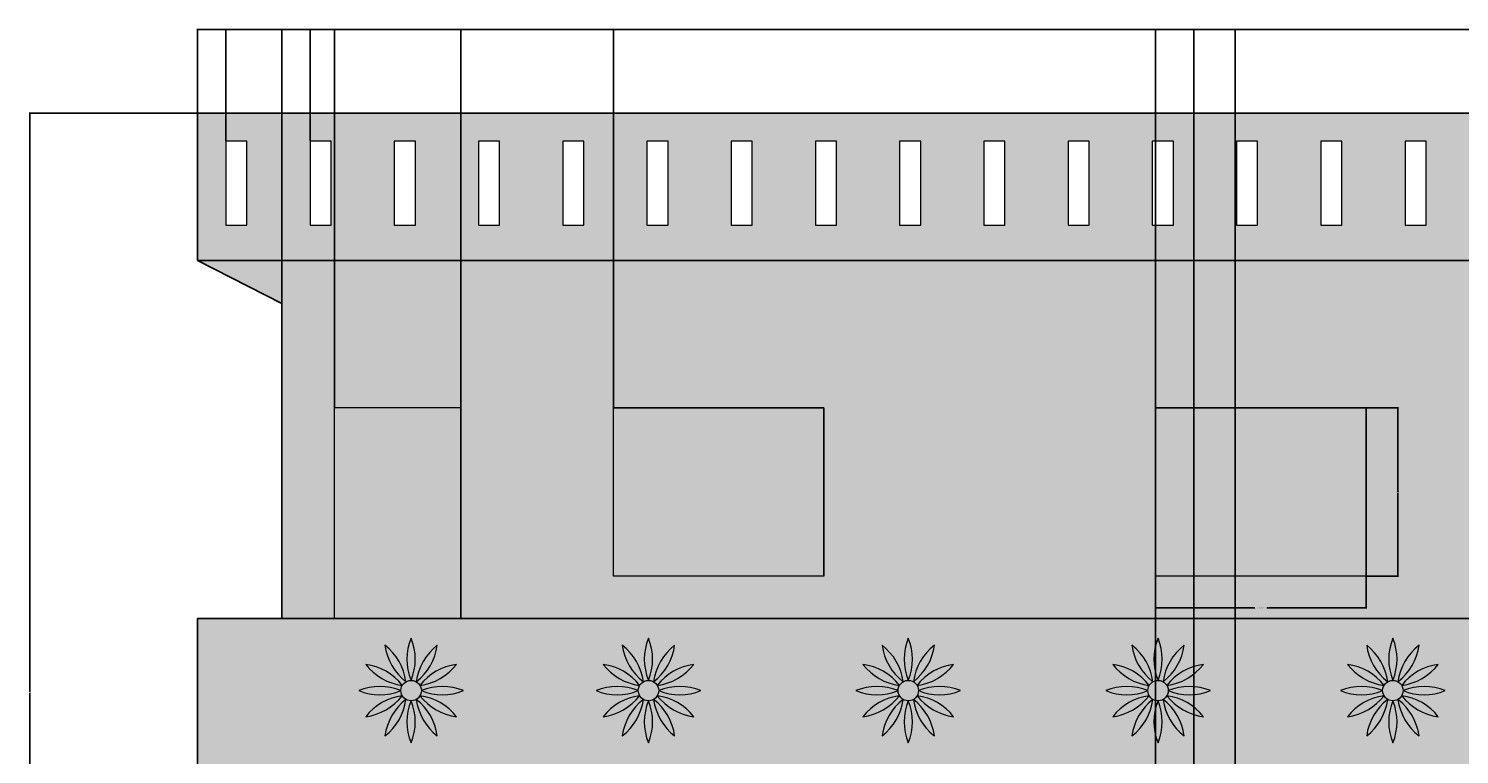
# Model space of a CAD drawing. Units: inches. Extents: x -43 to 1296, y -568 to 542.
# Tile 6 of 14: x -43 to 364, y 336 to 542. Entities that reach past the tile are written whole.
import ezdxf

# ---------------------------------------------------------------- set-up
doc = ezdxf.new("R2010")
doc.units = ezdxf.units.IN
doc.header["$MEASUREMENT"] = 0
for name, color, linetype, lineweight in [('A-ANNO-DIMS', 2, 'Continuous', 18), ('A-DOOR', 3, 'Continuous', 18), ('A-ELEV', 7, 'Continuous', 25), ('A-ELEV-OPEN-PATT', 13, 'Continuous', 13), ('A-ELEV-TRIM', 7, 'Continuous', 18), ('A-ELEV-TRIM-PATT', 4, 'Continuous', 13), ('A-GLAZ-ELEV', 4, 'Continuous', 18)]:
    doc.layers.add(name, color=color, linetype=linetype, lineweight=lineweight)
for name, color, linetype, lineweight, true_color in [('A-ELEV-BAND-PATT', 30, 'Continuous', 13, 0xf8991e), ('A-ELEV-WALL-PATT', 31, 'Continuous', 13, 0xfecc66), ('A-ROOF-PATT', 217, 'Continuous', 13, 0x93278f)]:
    doc.layers.add(name, color=color, linetype=linetype, lineweight=lineweight, true_color=true_color)
doc.styles.get("Standard").update_dxf_attribs({"font": 'arial.ttf'})
doc.dimstyles.get("Standard").update_dxf_attribs({"dimtxt": 0.18, "dimasz": 0.18, "dimexe": 0.18, "dimexo": 0.0625, "dimgap": 0.09, "dimtad": 0, "dimtih": 1, "dimtoh": 1, "dimdec": 0, "dimzin": 0, "dimdsep": 46, "dimlunit": 3, "dimtxsty": 'Standard', "dimcen": 0.09, "dimadec": 0, "dimazin": 0, "dimtfac": 1, "dimtdec": 0, "dimtofl": 0, "dimtmove": 0, "dimatfit": 3, "dimfxl": 1, "dimtolj": 1, "dimtzin": 0, "dimarcsym": 0})

# ---------------------------------------------------------------- blocks, each defined once
blk = doc.blocks.new('*U5')
for p, q in [((-3, 12), (-3, -12)), ((3, 12), (-3, 12)), ((3, -12), (3, 12)), ((-3, -12), (3, -12))]:
    blk.add_line(p, q)
blk = doc.blocks.new('*U6')
at = {"layer": 'A-ELEV-TRIM', "color": 0, "linetype": 'ByBlock', "lineweight": -2, "transparency": 16777216}
for p in [(0, 0), (24, 0), (48, 0), (72, 0), (96, 0), (120, 0), (144, 0), (168, 0), (192, 0), (216, 0), (240, 0), (264, 0), (288, 0), (312, 0), (336, 0), (360, 0), (384, 0)]:
    blk.add_blockref('*U5', p, dxfattribs=at)
blk = doc.blocks.new('*U9')
for centre, start, end in [((14.57, 0), 157.6165, 202.3835), ((-14.57, 0), 337.6165, 22.3835)]:
    blk.add_arc(centre, 15.76, start, end)
blk = doc.blocks.new('*U10')
at = {"layer": 'A-ELEV-TRIM', "color": 0, "linetype": 'ByBlock', "lineweight": -2, "transparency": 16777216}
for p, rotation in [((202.9, 361.45), 29.99999999999998), ((211.82, 361.45), 329.9999999999999), ((199.64, 358.19), 59.99999999999999), ((215.08, 358.19), 300), ((198.44, 353.73), 90), ((216.28, 353.73), 269.9999999999999), ((199.64, 349.27), 120), ((202.9, 346.01), 150), ((207.36, 344.81), 180), ((211.82, 346.01), 210), ((215.08, 349.27), 240)]:
    blk.add_blockref('*U9', p, dxfattribs=dict(at, rotation=rotation))
blk.add_blockref('*U9', (207.36, 362.65), dxfattribs=at)
blk = doc.blocks.new('*U11')
for centre, start, end in [((14.57, 0), 157.6165, 202.3835), ((-14.57, 0), 337.6165, 22.3835)]:
    blk.add_arc(centre, 15.76, start, end)
blk = doc.blocks.new('*U12')
at = {"layer": 'A-ELEV-TRIM', "color": 0, "linetype": 'ByBlock', "lineweight": -2, "transparency": 16777216}
for p, rotation in [((202.9, 361.45), 29.99999999999998), ((211.82, 361.45), 329.9999999999999), ((199.64, 358.19), 59.99999999999999), ((215.08, 358.19), 300), ((198.44, 353.73), 90), ((216.28, 353.73), 269.9999999999999), ((199.64, 349.27), 120), ((202.9, 346.01), 150), ((207.36, 344.81), 180), ((211.82, 346.01), 210), ((215.08, 349.27), 240)]:
    blk.add_blockref('*U11', p, dxfattribs=dict(at, rotation=rotation))
blk.add_blockref('*U11', (207.36, 362.65), dxfattribs=at)
blk = doc.blocks.new('*U13')
for centre, start, end in [((14.57, 0), 157.6165, 202.3835), ((-14.57, 0), 337.6165, 22.3835)]:
    blk.add_arc(centre, 15.76, start, end)
blk = doc.blocks.new('*U14')
at = {"layer": 'A-ELEV-TRIM', "color": 0, "linetype": 'ByBlock', "lineweight": -2, "transparency": 16777216}
for p, rotation in [((202.9, 361.45), 29.99999999999998), ((211.82, 361.45), 329.9999999999999), ((199.64, 358.19), 59.99999999999999), ((215.08, 358.19), 300), ((198.44, 353.73), 90), ((216.28, 353.73), 269.9999999999999), ((199.64, 349.27), 120), ((202.9, 346.01), 150), ((207.36, 344.81), 180), ((211.82, 346.01), 210), ((215.08, 349.27), 240)]:
    blk.add_blockref('*U13', p, dxfattribs=dict(at, rotation=rotation))
blk.add_blockref('*U13', (207.36, 362.65), dxfattribs=at)
blk = doc.blocks.new('*U15')
for centre, start, end in [((14.57, 0), 157.6165, 202.3835), ((-14.57, 0), 337.6165, 22.3835)]:
    blk.add_arc(centre, 15.76, start, end)
blk = doc.blocks.new('*U16')
at = {"layer": 'A-ELEV-TRIM', "color": 0, "linetype": 'ByBlock', "lineweight": -2, "transparency": 16777216}
for p, rotation in [((202.9, 361.45), 29.99999999999998), ((211.82, 361.45), 329.9999999999999), ((199.64, 358.19), 59.99999999999999), ((215.08, 358.19), 300), ((198.44, 353.73), 90), ((216.28, 353.73), 269.9999999999999), ((199.64, 349.27), 120), ((202.9, 346.01), 150), ((207.36, 344.81), 180), ((211.82, 346.01), 210), ((215.08, 349.27), 240)]:
    blk.add_blockref('*U15', p, dxfattribs=dict(at, rotation=rotation))
blk.add_blockref('*U15', (207.36, 362.65), dxfattribs=at)
blk = doc.blocks.new('*U17')
for centre, start, end in [((14.57, 0), 157.6165, 202.3835), ((-14.57, 0), 337.6165, 22.3835)]:
    blk.add_arc(centre, 15.76, start, end)
blk = doc.blocks.new('*U18')
at = {"layer": 'A-ELEV-TRIM', "color": 0, "linetype": 'ByBlock', "lineweight": -2, "transparency": 16777216}
for p, rotation in [((202.9, 361.45), 29.99999999999998), ((211.82, 361.45), 329.9999999999999), ((199.64, 358.19), 59.99999999999999), ((215.08, 358.19), 300), ((198.44, 353.73), 90), ((216.28, 353.73), 269.9999999999999), ((199.64, 349.27), 120), ((202.9, 346.01), 150), ((207.36, 344.81), 180), ((211.82, 346.01), 210), ((215.08, 349.27), 240)]:
    blk.add_blockref('*U17', p, dxfattribs=dict(at, rotation=rotation))
blk.add_blockref('*U17', (207.36, 362.65), dxfattribs=at)
blk = doc.blocks.new('WIN-ELEV-60x48')
for p, q in [((60, 48), (0, 48)), ((0, 0), (0, 48)), ((60, 0), (60, 48)), ((60, 0), (0, 0))]:
    blk.add_line(p, q)
blk = doc.blocks.new('*D52')
at = {"layer": 'A-ANNO-DIMS', "color": 0, "lineweight": -2, "transparency": 16777216}
for p, q in [((277.84, 386.23), (277.84, 377.11)), ((337.84, 386.23), (337.84, 377.11)), ((278.02, 377.29), (306.15, 377.29)), ((337.66, 377.29), (309.53, 377.29))]:
    blk.add_line(p, q, dxfattribs=at)
at = {"layer": 'A-ANNO-DIMS', "color": 0, "transparency": 16777216}
for points in [[(278.02, 377.32), (278.02, 377.26), (277.84, 377.29)], [(337.66, 377.32), (337.66, 377.26), (337.84, 377.29)]]:
    blk.add_solid(points, dxfattribs=at)
at = {"layer": 'Defpoints', "color": 0, "transparency": 16777216}
for p in [(277.84, 386.29), (337.84, 386.29), (337.84, 377.29)]:
    blk.add_point(p, dxfattribs=at)
at = {"layer": 'A-ANNO-DIMS', "color": 0, "transparency": 16777216, "insert": (307.84, 377.29), "char_height": 0.18, "attachment_point": 5}
blk.add_mtext('\\A1;UPPER WINDOW 5\'-0" TYP.', dxfattribs=at)
blk = doc.blocks.new('*D53')
at = {"layer": 'A-ANNO-DIMS', "color": 0, "lineweight": -2, "transparency": 16777216}
for p, q in [((337.91, 434.29), (347.02, 434.29)), ((346.84, 434.11), (346.84, 410.47)), ((346.84, 386.47), (346.84, 410.11)), ((337.91, 386.29), (347.02, 386.29))]:
    blk.add_line(p, q, dxfattribs=at)
at = {"layer": 'A-ANNO-DIMS', "color": 0, "transparency": 16777216}
for points in [[(346.81, 434.11), (346.87, 434.11), (346.84, 434.29)], [(346.81, 386.47), (346.87, 386.47), (346.84, 386.29)]]:
    blk.add_solid(points, dxfattribs=at)
at = {"layer": 'Defpoints', "color": 0, "transparency": 16777216}
for p in [(337.84, 434.29), (346.84, 434.29), (337.84, 386.29)]:
    blk.add_point(p, dxfattribs=at)
at = {"layer": 'A-ANNO-DIMS', "color": 0, "transparency": 16777216, "insert": (346.84, 410.29), "char_height": 0.18, "attachment_point": 5}
blk.add_mtext('\\A1;4\'-0" TYP.', dxfattribs=at)
blk = doc.blocks.new('*D61')
at = {"layer": 'A-ANNO-DIMS', "color": 0, "lineweight": -2, "transparency": 16777216}
for p, q in [((4.78, 518.29), (-43.14, 518.29)), ((-42.96, 518.11), (-42.96, 353.47)), ((-42.96, 188.47), (-42.96, 353.11)), ((-19.22, 188.29), (-43.14, 188.29))]:
    blk.add_line(p, q, dxfattribs=at)
at = {"layer": 'A-ANNO-DIMS', "color": 0, "transparency": 16777216}
for points in [[(-42.99, 518.11), (-42.93, 518.11), (-42.96, 518.29)], [(-42.99, 188.47), (-42.93, 188.47), (-42.96, 188.29)]]:
    blk.add_solid(points, dxfattribs=at)
at = {"layer": 'Defpoints', "color": 0, "transparency": 16777216}
for p in [(-42.96, 518.29), (4.84, 518.29), (-19.16, 188.29)]:
    blk.add_point(p, dxfattribs=at)
at = {"layer": 'A-ANNO-DIMS', "color": 0, "transparency": 16777216, "insert": (-42.96, 353.29), "char_height": 0.18, "attachment_point": 5}
blk.add_mtext('\\A1;27\'-6"', dxfattribs=at)
blk = doc.blocks.new('*D70')
at = {"layer": 'A-ANNO-DIMS', "color": 0, "lineweight": -2, "transparency": 16777216}
for p, q in [((277.84, 188.35), (277.84, 542.27)), ((288.75, 188.35), (288.75, 542.27)), ((278.02, 542.09), (282.89, 542.09)), ((288.57, 542.09), (283.69, 542.09))]:
    blk.add_line(p, q, dxfattribs=at)
at = {"layer": 'A-ANNO-DIMS', "color": 0, "transparency": 16777216}
for points in [[(278.02, 542.12), (278.02, 542.06), (277.84, 542.09)], [(288.57, 542.12), (288.57, 542.06), (288.75, 542.09)]]:
    blk.add_solid(points, dxfattribs=at)
at = {"layer": 'Defpoints', "color": 0, "transparency": 16777216}
for p in [(288.75, 542.09), (277.84, 188.29), (288.75, 188.29)]:
    blk.add_point(p, dxfattribs=at)
at = {"layer": 'A-ANNO-DIMS', "color": 0, "transparency": 16777216, "insert": (283.29, 542.09), "char_height": 0.18, "attachment_point": 5}
blk.add_mtext('\\A1;0\'-11"', dxfattribs=at)
blk = doc.blocks.new('*D71')
at = {"layer": 'A-ANNO-DIMS', "color": 0, "lineweight": -2, "transparency": 16777216}
for p, q in [((288.75, 235.13), (288.75, 542.27)), ((300.49, 239.65), (300.49, 542.27)), ((288.93, 542.09), (294.01, 542.09)), ((300.31, 542.09), (295.23, 542.09))]:
    blk.add_line(p, q, dxfattribs=at)
at = {"layer": 'A-ANNO-DIMS', "color": 0, "transparency": 16777216}
for points in [[(288.93, 542.12), (288.93, 542.06), (288.75, 542.09)], [(300.31, 542.12), (300.31, 542.06), (300.49, 542.09)]]:
    blk.add_solid(points, dxfattribs=at)
at = {"layer": 'Defpoints', "color": 0, "transparency": 16777216}
for p in [(300.49, 542.09), (300.49, 239.58), (288.75, 235.07)]:
    blk.add_point(p, dxfattribs=at)
at = {"layer": 'A-ANNO-DIMS', "color": 0, "transparency": 16777216, "insert": (294.62, 542.09), "char_height": 0.18, "attachment_point": 5}
blk.add_mtext('\\A1;0\'-11 1/2"', dxfattribs=at)
blk = doc.blocks.new('*D73')
at = {"layer": 'A-ANNO-DIMS', "color": 0, "lineweight": -2, "transparency": 16777216}
for p, q in [((4.84, 518.35), (4.84, 542.27)), ((412.84, 518.35), (412.84, 542.27)), ((5.02, 542.09), (208.44, 542.09)), ((412.66, 542.09), (209.24, 542.09))]:
    blk.add_line(p, q, dxfattribs=at)
at = {"layer": 'A-ANNO-DIMS', "color": 0, "transparency": 16777216}
for points in [[(5.02, 542.12), (5.02, 542.06), (4.84, 542.09)], [(412.66, 542.12), (412.66, 542.06), (412.84, 542.09)]]:
    blk.add_solid(points, dxfattribs=at)
at = {"layer": 'Defpoints', "color": 0, "transparency": 16777216}
for p in [(412.84, 542.09), (4.84, 518.29), (412.84, 518.29)]:
    blk.add_point(p, dxfattribs=at)
at = {"layer": 'A-ANNO-DIMS', "color": 0, "transparency": 16777216, "insert": (208.84, 542.09), "char_height": 0.18, "attachment_point": 5}
blk.add_mtext('\\A1;34\'-0"', dxfattribs=at)
blk = doc.blocks.new('*D74')
at = {"layer": 'A-ANNO-DIMS', "color": 0, "lineweight": -2, "transparency": 16777216}
for p, q in [((28.84, 476.35), (28.84, 542.27)), ((43.84, 434.35), (43.84, 542.27)), ((29.02, 542.09), (36.02, 542.09)), ((43.66, 542.09), (36.66, 542.09))]:
    blk.add_line(p, q, dxfattribs=at)
at = {"layer": 'A-ANNO-DIMS', "color": 0, "transparency": 16777216}
for points in [[(29.02, 542.12), (29.02, 542.06), (28.84, 542.09)], [(43.66, 542.12), (43.66, 542.06), (43.84, 542.09)]]:
    blk.add_solid(points, dxfattribs=at)
at = {"layer": 'Defpoints', "color": 0, "transparency": 16777216}
for p in [(43.84, 542.09), (28.84, 476.29), (43.84, 434.29)]:
    blk.add_point(p, dxfattribs=at)
at = {"layer": 'A-ANNO-DIMS', "color": 0, "transparency": 16777216, "insert": (36.34, 542.09), "char_height": 0.18, "attachment_point": 5}
blk.add_mtext('\\A1;1\'-3"', dxfattribs=at)
blk = doc.blocks.new('*D75')
at = {"layer": 'A-ANNO-DIMS', "color": 0, "lineweight": -2, "transparency": 16777216}
for p, q in [((43.84, 434.35), (43.84, 542.27)), ((79.84, 434.35), (79.84, 542.27)), ((44.02, 542.09), (61.51, 542.09)), ((79.66, 542.09), (62.17, 542.09))]:
    blk.add_line(p, q, dxfattribs=at)
at = {"layer": 'A-ANNO-DIMS', "color": 0, "transparency": 16777216}
for points in [[(44.02, 542.12), (44.02, 542.06), (43.84, 542.09)], [(79.66, 542.12), (79.66, 542.06), (79.84, 542.09)]]:
    blk.add_solid(points, dxfattribs=at)
at = {"layer": 'Defpoints', "color": 0, "transparency": 16777216}
for p in [(79.84, 542.09), (43.84, 434.29), (79.84, 434.29)]:
    blk.add_point(p, dxfattribs=at)
at = {"layer": 'A-ANNO-DIMS', "color": 0, "transparency": 16777216, "insert": (61.84, 542.09), "char_height": 0.18, "attachment_point": 5}
blk.add_mtext('\\A1;3\'-0"', dxfattribs=at)
blk = doc.blocks.new('*D76')
at = {"layer": 'A-ANNO-DIMS', "color": 0, "lineweight": -2, "transparency": 16777216}
for p, q in [((79.84, 434.35), (79.84, 542.27)), ((123.34, 434.35), (123.34, 542.27)), ((80.02, 542.09), (101.05, 542.09)), ((123.16, 542.09), (102.13, 542.09))]:
    blk.add_line(p, q, dxfattribs=at)
at = {"layer": 'A-ANNO-DIMS', "color": 0, "transparency": 16777216}
for points in [[(80.02, 542.12), (80.02, 542.06), (79.84, 542.09)], [(123.16, 542.12), (123.16, 542.06), (123.34, 542.09)]]:
    blk.add_solid(points, dxfattribs=at)
at = {"layer": 'Defpoints', "color": 0, "transparency": 16777216}
for p in [(123.34, 542.09), (79.84, 434.29), (123.34, 434.29)]:
    blk.add_point(p, dxfattribs=at)
at = {"layer": 'A-ANNO-DIMS', "color": 0, "transparency": 16777216, "insert": (101.59, 542.09), "char_height": 0.18, "attachment_point": 5}
blk.add_mtext('\\A1;3\'-7 1/2"', dxfattribs=at)
blk = doc.blocks.new('*D77')
at = {"layer": 'A-ANNO-DIMS', "color": 0, "lineweight": -2, "transparency": 16777216}
for p, q in [((123.34, 434.35), (123.34, 542.27)), ((277.84, 434.35), (277.84, 542.27)), ((123.52, 542.09), (199.92, 542.09)), ((277.66, 542.09), (201.26, 542.09))]:
    blk.add_line(p, q, dxfattribs=at)
at = {"layer": 'A-ANNO-DIMS', "color": 0, "transparency": 16777216}
for points in [[(123.52, 542.12), (123.52, 542.06), (123.34, 542.09)], [(277.66, 542.12), (277.66, 542.06), (277.84, 542.09)]]:
    blk.add_solid(points, dxfattribs=at)
at = {"layer": 'Defpoints', "color": 0, "transparency": 16777216}
for p in [(277.84, 542.09), (123.34, 434.29), (277.84, 434.29)]:
    blk.add_point(p, dxfattribs=at)
at = {"layer": 'A-ANNO-DIMS', "color": 0, "transparency": 16777216, "insert": (200.59, 542.09), "char_height": 0.18, "attachment_point": 5}
blk.add_mtext('\\A1;12\'-10 1/2"', dxfattribs=at)
blk = doc.blocks.new('*D78')
at = {"layer": 'A-ANNO-DIMS', "color": 0, "lineweight": -2, "transparency": 16777216}
for p, q in [((12.9, 510.38), (12.9, 542.27)), ((36.9, 510.38), (36.9, 542.27)), ((13.08, 542.09), (24.57, 542.09)), ((36.72, 542.09), (25.23, 542.09))]:
    blk.add_line(p, q, dxfattribs=at)
at = {"layer": 'A-ANNO-DIMS', "color": 0, "transparency": 16777216}
for points in [[(13.08, 542.12), (13.08, 542.06), (12.9, 542.09)], [(36.72, 542.12), (36.72, 542.06), (36.9, 542.09)]]:
    blk.add_solid(points, dxfattribs=at)
at = {"layer": 'Defpoints', "color": 0, "transparency": 16777216}
for p in [(36.9, 542.09), (12.9, 510.31), (36.9, 510.31)]:
    blk.add_point(p, dxfattribs=at)
at = {"layer": 'A-ANNO-DIMS', "color": 0, "transparency": 16777216, "insert": (24.9, 542.09), "char_height": 0.18, "attachment_point": 5}
blk.add_mtext('\\A1;2\'-0"', dxfattribs=at)

msp = doc.modelspace()

# ---------------------------------------------------------------- hatches: boundary and pattern name
at = {"layer": 'A-ELEV-BAND-PATT'}
h = msp.add_hatch(color=256, dxfattribs=at)
h.dxf.hatch_style = 1
h.paths.add_polyline_path([(412.84, 374.29), (4.84, 374.29), (4.84, 332.29), (412.84, 332.29)])
h.paths.add_polyline_path([(222.28, 353.73, -0.197856), (210.28, 353.73, -0.131652), (209.89, 352.27, -0.197856), (220.28, 346.27, -0.197856), (209.89, 352.27, -0.131652), (208.82, 351.2, -0.197856), (214.82, 340.81, -0.197856), (208.82, 351.2, -0.131652), (207.36, 350.81, -0.197856), (207.36, 338.81, -0.197856), (207.36, 350.81, -0.131652), (205.9, 351.2, -0.197856), (199.9, 340.81, -0.197856), (205.9, 351.2, -0.131652), (204.83, 352.27, -0.197856), (194.44, 346.27, -0.197856), (204.83, 352.27, -0.131652), (204.44, 353.73, -0.197856), (192.44, 353.73, -0.197856), (204.44, 353.73, -0.131652), (204.83, 355.19, -0.197856), (194.44, 361.19, -0.197856), (204.83, 355.19, -0.131652), (205.9, 356.25, -0.197856), (199.9, 366.65, -0.197856), (205.9, 356.25, -0.131652), (207.36, 356.65, -0.197856), (207.36, 368.65, -0.197856), (207.36, 356.65, -0.131652), (208.82, 356.25, -0.197856), (214.82, 366.65, -0.197856), (208.82, 356.25, -0.131652), (209.89, 355.19, -0.197856), (220.28, 361.19, -0.197856), (209.89, 355.19, -0.131652), (210.28, 353.73, -0.197856)], flags=16)
h.paths.add_polyline_path([(263.61, 353.73, -0.197856), (275.61, 353.73, -0.131652), (276, 355.19, -0.197856), (265.61, 361.19, -0.197856), (276, 355.19, -0.131652), (277.07, 356.25, -0.197856), (271.07, 366.65, -0.197856), (277.07, 356.25, -0.131652), (278.53, 356.65, -0.197856), (278.53, 368.65, -0.197856), (278.53, 356.65, -0.131652), (279.99, 356.25, -0.197856), (285.99, 366.65, -0.197856), (279.99, 356.25, -0.131652), (281.06, 355.19, -0.197856), (291.45, 361.19, -0.197856), (281.06, 355.19, -0.131652), (281.45, 353.73, -0.197856), (293.45, 353.73, -0.197856), (281.45, 353.73, -0.131652), (281.06, 352.27, -0.197856), (291.45, 346.27, -0.197856), (281.06, 352.27, -0.131652), (279.99, 351.2, -0.197856), (285.99, 340.81, -0.197856), (279.99, 351.2, -0.131652), (278.53, 350.81, -0.197856), (278.53, 338.81, -0.197856), (278.53, 350.81, -0.131652), (277.07, 351.2, -0.197856), (271.07, 340.81, -0.197856), (277.07, 351.2, -0.131652), (276, 352.27, -0.197856), (265.61, 346.27, -0.197856), (276, 352.27, -0.131652), (275.61, 353.73, -0.197856)], flags=16)
h.paths.add_polyline_path([(330.52, 353.73, -0.197856), (342.52, 353.73, -0.131652), (342.91, 355.19, -0.197856), (332.52, 361.19, -0.197856), (342.91, 355.19, -0.131652), (343.98, 356.25, -0.197856), (337.98, 366.65, -0.197856), (343.98, 356.25, -0.131652), (345.44, 356.65, -0.197856), (345.44, 368.65, -0.197856), (345.44, 356.65, -0.131652), (346.9, 356.25, -0.197856), (352.9, 366.65, -0.197856), (346.9, 356.25, -0.131652), (347.97, 355.19, -0.197856), (358.36, 361.19, -0.197856), (347.97, 355.19, -0.131652), (348.36, 353.73, -0.197856), (360.36, 353.73, -0.197856), (348.36, 353.73, -0.131652), (347.97, 352.27, -0.197856), (358.36, 346.27, -0.197856), (347.97, 352.27, -0.131652), (346.9, 351.2, -0.197856), (352.9, 340.81, -0.197856), (346.9, 351.2, -0.131652), (345.44, 350.81, -0.197856), (345.44, 338.81, -0.197856), (345.44, 350.81, -0.131652), (343.98, 351.2, -0.197856), (337.98, 340.81, -0.197856), (343.98, 351.2, -0.131652), (342.91, 352.27, -0.197856), (332.52, 346.27, -0.197856), (342.91, 352.27, -0.131652), (342.52, 353.73, -0.197856)], flags=16)
h.paths.add_polyline_path([(148.25, 353.73, -0.197856), (136.25, 353.73, -0.131652), (135.85, 352.27, -0.197856), (146.25, 346.27, -0.197856), (135.85, 352.27, -0.131652), (134.79, 351.2, -0.197856), (140.79, 340.81, -0.197856), (134.79, 351.2, -0.131652), (133.33, 350.81, -0.197856), (133.33, 338.81, -0.197856), (133.33, 350.81, -0.131652), (131.87, 351.2, -0.197856), (125.87, 340.81, -0.197856), (131.87, 351.2, -0.131652), (130.8, 352.27, -0.197856), (120.41, 346.27, -0.197856), (130.8, 352.27, -0.131652), (130.41, 353.73, -0.197856), (118.41, 353.73, -0.197856), (130.41, 353.73, -0.131652), (130.8, 355.19, -0.197856), (120.41, 361.19, -0.197856), (130.8, 355.19, -0.131652), (131.87, 356.25, -0.197856), (125.87, 366.65, -0.197856), (131.87, 356.25, -0.131652), (133.33, 356.65, -0.197856), (133.33, 368.65, -0.197856), (133.33, 356.65, -0.131652), (134.79, 356.25, -0.197856), (140.79, 366.65, -0.197856), (134.79, 356.25, -0.131652), (135.85, 355.19, -0.197856), (146.25, 361.19, -0.197856), (135.85, 355.19, -0.131652), (136.25, 353.73, -0.197856)], flags=16)
h.paths.add_polyline_path([(80.61, 353.73, -0.197856), (68.61, 353.73, -0.131652), (68.22, 352.27, -0.197856), (78.61, 346.27, -0.197856), (68.22, 352.27, -0.131652), (67.15, 351.2, -0.197856), (73.15, 340.81, -0.197856), (67.15, 351.2, -0.131652), (65.69, 350.81, -0.197856), (65.69, 338.81, -0.197856), (65.69, 350.81, -0.131652), (64.23, 351.2, -0.197856), (58.23, 340.81, -0.197856), (64.23, 351.2, -0.131652), (63.16, 352.27, -0.197856), (52.77, 346.27, -0.197856), (63.16, 352.27, -0.131652), (62.77, 353.73, -0.197856), (50.77, 353.73, -0.197856), (62.77, 353.73, -0.131652), (63.16, 355.19, -0.197856), (52.77, 361.19, -0.197856), (63.16, 355.19, -0.131652), (64.23, 356.25, -0.197856), (58.23, 366.65, -0.197856), (64.23, 356.25, -0.131652), (65.69, 356.65, -0.197856), (65.69, 368.65, -0.197856), (65.69, 356.65, -0.131652), (67.15, 356.25, -0.197856), (73.15, 366.65, -0.197856), (67.15, 356.25, -0.131652), (68.22, 355.19, -0.197856), (78.61, 361.19, -0.197856), (68.22, 355.19, -0.131652), (68.61, 353.73, -0.197856)], flags=16)
at = {"layer": 'A-ELEV-OPEN-PATT'}
h = msp.add_hatch(color=256, dxfattribs=at)
h.dxf.hatch_style = 1
h.paths.add_polyline_path([(79.84, 434.29), (43.84, 434.29), (43.84, 374.29), (79.84, 374.29)])
h.paths.add_polyline_path([(183.34, 434.29), (123.34, 434.29), (123.34, 386.29), (183.34, 386.29)])
h.paths.add_polyline_path([(337.84, 434.29), (277.84, 434.29), (277.84, 386.29), (337.84, 386.29)])
h.paths.add_polyline_path([(79.84, 290.29), (43.84, 290.29), (43.84, 248.29), (79.84, 248.29)])
h.paths.add_polyline_path([(183.34, 290.29), (123.34, 290.29), (123.34, 248.29), (183.34, 248.29)])
h.paths.add_polyline_path([(337.84, 290.29), (277.84, 290.29), (277.84, 248.29), (277.84, 230.87), (323.14, 248.29), (337.84, 242.64), (337.84, 248.29)])
h.paths.add_polyline_path([(1016.13, 374.59), (980.13, 374.59), (980.13, 290.59), (1016.13, 290.59)])
h.paths.add_polyline_path([(1016.13, 230.59), (980.13, 230.59), (980.13, 146.59), (1016.13, 146.59)])
h.paths.add_polyline_path([(833.13, 374.59), (824.13, 374.59), (824.13, 326.59), (833.13, 326.59)])
h.paths.add_polyline_path([(833.13, 230.59), (824.13, 230.59), (824.13, 182.59), (833.13, 182.59)])
at = {"layer": 'A-ELEV-TRIM-PATT'}
h = msp.add_hatch(color=256, dxfattribs=at)
h.dxf.hatch_style = 1
h.paths.add_polyline_path([(222.28, 353.73, -0.197856), (210.28, 353.73, -0.131652), (209.89, 352.27, -0.197856), (220.28, 346.27, -0.197856), (209.89, 352.27, -0.131652), (208.82, 351.2, -0.197856), (214.82, 340.81, -0.197856), (208.82, 351.2, -0.131652), (207.36, 350.81, -0.197856), (207.36, 338.81, -0.197856), (207.36, 350.81, -0.131652), (205.9, 351.2, -0.197856), (199.9, 340.81, -0.197856), (205.9, 351.2, -0.131652), (204.83, 352.27, -0.197856), (194.44, 346.27, -0.197856), (204.83, 352.27, -0.131652), (204.44, 353.73, -0.197856), (192.44, 353.73, -0.197856), (204.44, 353.73, -0.131652), (204.83, 355.19, -0.197856), (194.44, 361.19, -0.197856), (204.83, 355.19, -0.131652), (205.9, 356.25, -0.197856), (199.9, 366.65, -0.197856), (205.9, 356.25, -0.131652), (207.36, 356.65, -0.197856), (207.36, 368.65, -0.197856), (207.36, 356.65, -0.131652), (208.82, 356.25, -0.197856), (214.82, 366.65, -0.197856), (208.82, 356.25, -0.131652), (209.89, 355.19, -0.197856), (220.28, 361.19, -0.197856), (209.89, 355.19, -0.131652), (210.28, 353.73, -0.197856)])
h.paths.add_polyline_path([(293.45, 353.73, -0.197856), (281.45, 353.73, -0.131652), (281.06, 352.27, -0.197856), (291.45, 346.27, -0.197856), (281.06, 352.27, -0.131652), (279.99, 351.2, -0.197856), (285.99, 340.81, -0.197856), (279.99, 351.2, -0.131652), (278.53, 350.81, -0.197856), (278.53, 338.81, -0.197856), (278.53, 350.81, -0.131652), (277.07, 351.2, -0.197856), (271.07, 340.81, -0.197856), (277.07, 351.2, -0.131652), (276, 352.27, -0.197856), (265.61, 346.27, -0.197856), (276, 352.27, -0.131652), (275.61, 353.73, -0.197856), (263.61, 353.73, -0.197856), (275.61, 353.73, -0.131652), (276, 355.19, -0.197856), (265.61, 361.19, -0.197856), (276, 355.19, -0.131652), (277.07, 356.25, -0.197856), (271.07, 366.65, -0.197856), (277.07, 356.25, -0.131652), (278.53, 356.65, -0.197856), (278.53, 368.65, -0.197856), (278.53, 356.65, -0.131652), (279.99, 356.25, -0.197856), (285.99, 366.65, -0.197856), (279.99, 356.25, -0.131652), (281.06, 355.19, -0.197856), (291.45, 361.19, -0.197856), (281.06, 355.19, -0.131652), (281.45, 353.73, -0.197856)])
h.paths.add_polyline_path([(342.52, 353.73, 1), (348.36, 353.73, 1)])
h.paths.add_polyline_path([(136.25, 353.73, 1), (130.41, 353.73, 1)])
h.paths.add_polyline_path([(68.61, 353.73, 1), (62.77, 353.73, 1)])
h.paths.add_polyline_path([(58.23, 366.65, 0.197856), (64.23, 356.25, 0.197856)])
h.paths.add_polyline_path([(65.69, 368.65, 0.197856), (65.69, 356.65, 0.197856)])
h.paths.add_polyline_path([(73.15, 366.65, 0.197856), (67.15, 356.25, 0.197856)])
h.paths.add_polyline_path([(78.61, 361.19, 0.197856), (68.22, 355.19, 0.197856)])
h.paths.add_polyline_path([(80.61, 353.73, 0.197856), (68.61, 353.73, 0.197856)])
h.paths.add_polyline_path([(68.22, 352.27, 0.197856), (78.61, 346.27, 0.197856)])
h.paths.add_polyline_path([(67.15, 351.2, 0.197856), (73.15, 340.81, 0.197856)])
h.paths.add_polyline_path([(65.69, 350.81, 0.197856), (65.69, 338.81, 0.197856)])
h.paths.add_polyline_path([(64.23, 351.2, 0.197856), (58.23, 340.81, 0.197856)])
h.paths.add_polyline_path([(63.16, 352.27, 0.197856), (52.77, 346.27, 0.197856)])
h.paths.add_polyline_path([(62.77, 353.73, 0.197856), (50.77, 353.73, 0.197856)])
h.paths.add_polyline_path([(52.77, 361.19, 0.197856), (63.16, 355.19, 0.197856)])
h.paths.add_polyline_path([(130.8, 352.27, 0.197856), (120.41, 346.27, 0.197856)])
h.paths.add_polyline_path([(130.41, 353.73, 0.197856), (118.41, 353.73, 0.197856)])
h.paths.add_polyline_path([(120.41, 361.19, 0.197856), (130.8, 355.19, 0.197856)])
h.paths.add_polyline_path([(125.87, 366.65, 0.197856), (131.87, 356.25, 0.197856)])
h.paths.add_polyline_path([(133.33, 368.65, 0.197856), (133.33, 356.65, 0.197856)])
h.paths.add_polyline_path([(140.79, 366.65, 0.197856), (134.79, 356.25, 0.197856)])
h.paths.add_polyline_path([(146.25, 361.19, 0.197856), (135.85, 355.19, 0.197856)])
h.paths.add_polyline_path([(136.25, 353.73, 0.197856), (148.25, 353.73, 0.197856)])
h.paths.add_polyline_path([(135.85, 352.27, 0.197856), (146.25, 346.27, 0.197856)])
h.paths.add_polyline_path([(134.79, 351.2, 0.197856), (140.79, 340.81, 0.197856)])
h.paths.add_polyline_path([(133.33, 350.81, 0.197856), (133.33, 338.81, 0.197856)])
h.paths.add_polyline_path([(131.87, 351.2, 0.197856), (125.87, 340.81, 0.197856)])
h.paths.add_polyline_path([(348.36, 353.73, 0.197856), (360.36, 353.73, 0.197856)])
h.paths.add_polyline_path([(358.36, 361.19, 0.197856), (347.97, 355.19, 0.197856)])
h.paths.add_polyline_path([(352.9, 366.65, 0.197856), (346.9, 356.25, 0.197856)])
h.paths.add_polyline_path([(345.44, 368.65, 0.197856), (345.44, 356.65, 0.197856)])
h.paths.add_polyline_path([(337.98, 366.65, 0.197856), (343.98, 356.25, 0.197856)])
h.paths.add_polyline_path([(332.52, 361.19, 0.197856), (342.91, 355.19, 0.197856)])
h.paths.add_polyline_path([(342.52, 353.73, 0.197856), (330.52, 353.73, 0.197856)])
h.paths.add_polyline_path([(342.91, 352.27, 0.197856), (332.52, 346.27, 0.197856)])
h.paths.add_polyline_path([(343.98, 351.2, 0.197856), (337.98, 340.81, 0.197856)])
h.paths.add_polyline_path([(345.44, 350.81, 0.197856), (345.44, 338.81, 0.197856)])
h.paths.add_polyline_path([(346.9, 351.2, 0.197856), (352.9, 340.81, 0.197856)])
h.paths.add_polyline_path([(347.97, 352.27, 0.197856), (358.36, 346.27, 0.197856)])
at = {"layer": 'A-ELEV-WALL-PATT'}
h = msp.add_hatch(color=256, dxfattribs=at)
h.dxf.hatch_style = 1
h.paths.add_polyline_path([(388.84, 476.29), (28.84, 476.29), (28.84, 374.29), (43.84, 374.29), (43.84, 434.29), (79.84, 434.29), (79.84, 374.29), (388.84, 374.29)])
h.paths.add_polyline_path([(123.34, 434.29), (183.34, 434.29), (183.34, 386.29), (123.34, 386.29)], flags=16)
h.paths.add_polyline_path([(277.84, 434.29), (337.84, 434.29), (337.84, 386.29), (277.84, 386.29)], flags=16)
at = {"layer": 'A-ROOF-PATT'}
h = msp.add_hatch(color=256, dxfattribs=at)
h.dxf.hatch_style = 1
h.paths.add_polyline_path([(412.84, 518.29), (388.84, 518.29), (28.84, 518.29), (4.84, 518.29), (4.84, 476.29), (412.84, 476.29)])
h.paths.add_polyline_path([(204.9, 510.31), (210.9, 510.31), (210.9, 486.31), (204.9, 486.31)], flags=16)
h.paths.add_polyline_path([(186.9, 486.31), (180.9, 486.31), (180.9, 510.31), (186.9, 510.31)], flags=16)
h.paths.add_polyline_path([(228.9, 510.31), (234.9, 510.31), (234.9, 486.31), (228.9, 486.31)], flags=16)
h.paths.add_polyline_path([(162.9, 486.31), (156.9, 486.31), (156.9, 510.31), (162.9, 510.31)], flags=16)
h.paths.add_polyline_path([(252.9, 510.31), (258.9, 510.31), (258.9, 486.31), (252.9, 486.31)], flags=16)
h.paths.add_polyline_path([(138.9, 486.31), (132.9, 486.31), (132.9, 510.31), (138.9, 510.31)], flags=16)
h.paths.add_polyline_path([(276.9, 510.31), (282.9, 510.31), (282.9, 486.31), (276.9, 486.31)], flags=16)
h.paths.add_polyline_path([(114.9, 486.31), (108.9, 486.31), (108.9, 510.31), (114.9, 510.31)], flags=16)
h.paths.add_polyline_path([(300.9, 510.31), (306.9, 510.31), (306.9, 486.31), (300.9, 486.31)], flags=16)
h.paths.add_polyline_path([(90.9, 486.31), (84.9, 486.31), (84.9, 510.31), (90.9, 510.31)], flags=16)
h.paths.add_polyline_path([(324.9, 510.31), (330.9, 510.31), (330.9, 486.31), (324.9, 486.31)], flags=16)
h.paths.add_polyline_path([(66.9, 486.31), (60.9, 486.31), (60.9, 510.31), (66.9, 510.31)], flags=16)
h.paths.add_polyline_path([(348.9, 510.31), (354.9, 510.31), (354.9, 486.31), (348.9, 486.31)], flags=16)
h.paths.add_polyline_path([(42.9, 486.31), (36.9, 486.31), (36.9, 510.31), (42.9, 510.31)], flags=16)
h.paths.add_polyline_path([(372.9, 510.31), (378.9, 510.31), (378.9, 486.31), (372.9, 486.31)], flags=16)
h.paths.add_polyline_path([(18.9, 486.31), (12.9, 486.31), (12.9, 510.31), (18.9, 510.31)], flags=16)
h.paths.add_polyline_path([(396.9, 510.31), (402.9, 510.31), (402.9, 486.31), (396.9, 486.31)], flags=16)
h = msp.add_hatch(color=256, dxfattribs=at)
h.dxf.hatch_style = 1
h.paths.add_polyline_path([(28.84, 476.29), (4.84, 476.29), (28.84, 464)])
h.paths.add_polyline_path([(412.84, 476.29), (388.84, 476.29), (388.84, 467.84)])

# ---------------------------------------------------------------- linework, layer by layer
at = {"layer": 'A-DOOR'}
for p, q in [((43.84, 374.29), (43.84, 434.29)), ((79.84, 434.29), (43.84, 434.29)), ((79.84, 374.29), (79.84, 434.29))]:
    msp.add_line(p, q, dxfattribs=at)
for points in [[(43.84, 374.29), (43.84, 434.29)], [(79.84, 434.29), (79.84, 374.29)]]:
    msp.add_lwpolyline(points, dxfattribs=at)
at = {"layer": 'A-ELEV'}
for p, q in [((4.84, 518.29), (28.84, 518.29)), ((4.84, 476.29), (4.84, 518.29)), ((388.84, 518.29), (28.84, 518.29)), ((412.84, 476.29), (4.84, 476.29)), ((4.84, 476.29), (28.84, 464)), ((28.84, 374.29), (28.84, 476.29)), ((412.84, 374.29), (4.84, 374.29)), ((4.84, 332.29), (4.84, 374.29))]:
    msp.add_line(p, q, dxfattribs=at)
at = {"layer": 'A-ELEV-TRIM'}
for centre in [(65.69, 353.73), (133.33, 353.73), (207.36, 353.73), (278.53, 353.73), (345.44, 353.73)]:
    msp.add_circle(centre, 2.92, dxfattribs=at)
at = {"layer": 'A-GLAZ-ELEV'}
for points in [[(123.34, 434.29), (183.34, 434.29), (183.34, 386.29), (123.34, 386.29)], [(277.84, 434.29), (337.84, 434.29), (337.84, 386.29), (277.84, 386.29)]]:
    msp.add_lwpolyline(points, close=True, dxfattribs=at)

# ---------------------------------------------------------------- block references
at = {"layer": 'A-ELEV-TRIM'}
for name, p in [('*U6', (15.9, 498.31)), ('*U18', (-141.67, 0)), ('*U12', (-74.03, 0)), ('*U10', (0, 0)), ('*U14', (71.17, 0)), ('*U16', (138.08, 0))]:
    msp.add_blockref(name, p, dxfattribs=at)
at = {"layer": 'A-GLAZ-ELEV'}
for p in [(123.34, 386.29), (277.84, 386.29)]:
    msp.add_blockref('WIN-ELEV-60x48', p, dxfattribs=at)

# ---------------------------------------------------------------- dimensions: what is measured, and where the dimension line sits
at = {"layer": 'A-ANNO-DIMS'}
for base, p1, p2, picture, middle in [((412.84, 542.09), (4.84, 518.29), (412.84, 518.29), '*D73', (208.84, 542.09)), ((36.9, 542.09), (12.9, 510.31), (36.9, 510.31), '*D78', (24.9, 542.09)), ((43.84, 542.09), (28.84, 476.29), (43.84, 434.29), '*D74', (36.34, 542.09)), ((79.84, 542.09), (43.84, 434.29), (79.84, 434.29), '*D75', (61.84, 542.09)), ((123.34, 542.09), (79.84, 434.29), (123.34, 434.29), '*D76', (101.59, 542.09)), ((277.84, 542.09), (123.34, 434.29), (277.84, 434.29), '*D77', (200.59, 542.09)), ((288.75, 542.09), (277.84, 188.29), (288.75, 188.29), '*D70', (283.29, 542.09)), ((300.49, 542.09), (288.75, 235.07), (300.49, 239.58), '*D71', (294.62, 542.09))]:
    dim = msp.add_linear_dim(base=base, p1=p1, p2=p2, dimstyle='Standard', override={"dimdec": 1, "dimlfac": 1, "dimrnd": 0, "dimzin": 1, "dimdsep": 46, "dimlunit": 4, "dimfrac": 2}, dxfattribs=at)
    dim.commit()
    dim.dimension.update_dxf_attribs({"geometry": picture, "text_midpoint": middle})
dim = msp.add_linear_dim(base=(-42.96, 518.29), p1=(-19.16, 188.29), p2=(4.84, 518.29), angle=90, dimstyle='Standard', override={"dimdec": 1, "dimlfac": 1, "dimrnd": 0, "dimzin": 1, "dimdsep": 46, "dimlunit": 4, "dimfrac": 2}, dxfattribs=at)
dim.commit()
dim.dimension.update_dxf_attribs({"geometry": '*D61', "text_midpoint": (-42.96, 353.29)})
dim = msp.add_linear_dim(base=(346.84, 434.29), p1=(337.84, 386.29), p2=(337.84, 434.29), angle=90, text='<> TYP.', dimstyle='Standard', override={"dimdec": 1, "dimlfac": 1, "dimrnd": 0, "dimzin": 1, "dimdsep": 46, "dimlunit": 4, "dimfrac": 2}, dxfattribs=at)
dim.commit()
dim.dimension.update_dxf_attribs({"geometry": '*D53', "text_midpoint": (346.84, 410.29)})
dim = msp.add_linear_dim(base=(337.84, 377.29), p1=(277.84, 386.29), p2=(337.84, 386.29), text='UPPER WINDOW <> TYP.', dimstyle='Standard', override={"dimdec": 1, "dimlfac": 1, "dimrnd": 0, "dimzin": 1, "dimdsep": 46, "dimlunit": 4, "dimfrac": 2}, dxfattribs=at)
dim.commit()
dim.dimension.update_dxf_attribs({"geometry": '*D52', "text_midpoint": (307.84, 377.29)})

doc.saveas('drawing.dxf')
